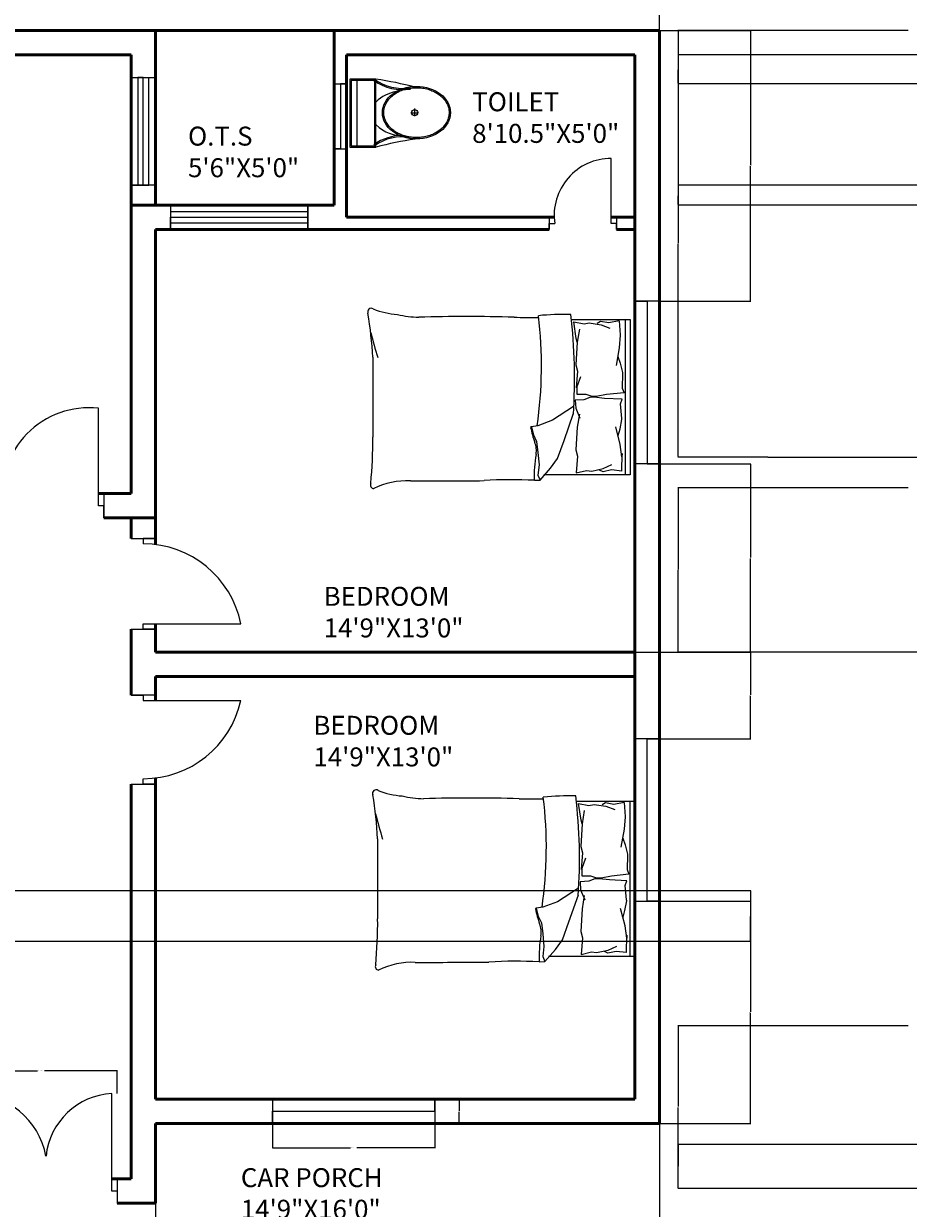
# Model space of a CAD drawing. Units: inches. Extents: x 2215 to 3724, y 1009 to 2124.
# Tile 6 of 11: x 2636 to 2963, y 1313 to 1750. Entities that reach past the tile are written whole.
import ezdxf

# ---------------------------------------------------------------- set-up
doc = ezdxf.new("R2010")
doc.units = ezdxf.units.IN
for name, color, linetype, lineweight in [('A-ANNO-DIMS', 2, 'Continuous', 18), ('A-ANNO-SYMB', 7, 'Continuous', 25), ('A-AREA-IDEN', 7, 'Continuous', 18), ('A-DOOR', 3, 'Continuous', 25), ('A-FLOR-FIXT', 9, 'Continuous', 18), ('A-FURN', 8, 'Continuous', 18), ('A-GLAZ', 4, 'Continuous', 18), ('A-WALL', 7, 'Continuous', 50)]:
    doc.layers.add(name, color=color, linetype=linetype, lineweight=lineweight)
doc.styles.get("Standard").update_dxf_attribs({"font": 'arial.ttf'})
doc.dimstyles.get("Standard").update_dxf_attribs({"dimtxt": 0.18, "dimasz": 0.18, "dimexe": 0.18, "dimexo": 0.0625, "dimgap": 0.09, "dimtad": 0, "dimtih": 1, "dimtoh": 1, "dimdec": 4, "dimzin": 0, "dimdsep": 46, "dimtxsty": 'Standard', "dimcen": 0.09, "dimadec": 0, "dimazin": 0, "dimtfac": 1, "dimtdec": 4, "dimtofl": 0, "dimtmove": 0, "dimatfit": 3, "dimfxl": 1, "dimtolj": 1, "dimtzin": 0, "dimarcsym": 0})

# ---------------------------------------------------------------- blocks, each defined once
blk = doc.blocks.new('A$C31115884')
for p, q in [((283.1, 497.7), (223.4, 497.7)), ((257.5, 466.4), (257.5, 523.2)), ((0, 200), (0, 0)), ((520, 200), (0, 200)), ((10, 190), (10, 10)), ((510, 190), (10, 190)), ((510, 10), (510, 190)), ((520, 0), (520, 200)), ((510, 54.5), (0, 54.5)), ((10, 10), (510, 10)), ((0, 0), (520, 0))]:
    blk.add_line(p, q)
blk.add_circle((255.6, 496.4), 23.6)
for centre, radius, start, end in [((2777.7, -204.6), 2807, 165.4549, 171.71327), ((-294.5, 403.3), 364.7, 324.20913, 9.34987), ((-294.5, 403.3), 374.7, 324.20913, 9.34987), ((805.8, 403.3), 364.7, 170.65013, 215.79087), ((3237, 905), 2807, 188.28673, 194.5451), ((139.5, 406.2), 293.5, 315.84364, 2.65635), ((805.8, 403.3), 374.7, 179.20365, 215.79087), ((383.6, 406.2), 293.5, 190.27735, 224.15636)]:
    blk.add_arc(centre, radius, start, end)
blk.add_ellipse((256.2, 509.9), major_axis=(0, -260.7), ratio=0.772727)
blk.add_open_spline([(256.2, 259.2), (263.1, 259.2), (270, 259.7), (287.8, 262.3), (298.7, 265.1), (319.9, 273.1), (330.2, 278.4), (350.1, 291.1), (359.7, 298.7), (377.7, 315.9), (386.2, 325.5), (401.7, 346.6), (408.8, 358.1), (421.3, 382.5), (426.8, 395.5), (435.9, 422.4), (439.5, 436.4), (444.8, 465.1), (446.5, 479.7), (447.9, 509.2), (447.6, 524), (445, 553.3), (442.7, 567.8), (436.3, 596), (432.1, 609.7), (421.9, 636), (416, 648.6), (402.5, 672.1), (395, 683), (378.6, 703), (369.8, 712.1), (351.1, 728), (341.3, 734.8), (320.9, 746.2), (310.4, 750.7), (288.9, 757.3), (278, 759.4), (256, 761), (245, 760.6), (223.1, 757.2), (212.3, 754.3), (191.1, 746.1), (180.8, 740.7), (160.9, 727.8), (151.4, 720.1), (133.5, 702.7), (125.1, 693), (109.6, 671.7), (102.6, 660.2), (90.2, 635.7), (84.9, 622.7), (76, 595.6), (72.4, 581.6), (67.2, 552.9), (65.6, 538.2), (64.4, 508.8), (64.8, 494), (67.5, 464.7), (69.9, 450.2), (76.6, 422), (80.8, 408.3), (91.1, 382.2), (97.2, 369.7), (110.8, 346.3), (118.4, 335.4), (134.8, 315.6), (143.7, 306.7), (162.4, 290.9), (172.3, 284.2), (192.8, 273), (203.3, 268.6), (224.8, 262.2), (235.8, 260.2), (249.9, 259.3), (253, 259.2), (256.2, 259.2)], degree=3, knots=[0, 0, 0, 0, 0.110105, 0.110105, 0.285049, 0.285049, 0.459994, 0.459994, 0.634938, 0.634938, 0.809882, 0.809882, 0.984827, 0.984827, 1.159771, 1.159771, 1.334715, 1.334715, 1.50966, 1.50966, 1.684604, 1.684604, 1.859549, 1.859549, 2.034493, 2.034493, 2.209437, 2.209437, 2.384382, 2.384382, 2.559326, 2.559326, 2.73427, 2.73427, 2.909215, 2.909215, 3.084159, 3.084159, 3.259103, 3.259103, 3.434048, 3.434048, 3.608992, 3.608992, 3.783936, 3.783936, 3.958881, 3.958881, 4.133825, 4.133825, 4.30877, 4.30877, 4.483714, 4.483714, 4.658658, 4.658658, 4.833603, 4.833603, 5.008547, 5.008547, 5.183491, 5.183491, 5.358436, 5.358436, 5.53338, 5.53338, 5.708324, 5.708324, 5.883269, 5.883269, 6.058213, 6.058213, 6.233158, 6.233158, 6.283185, 6.283185, 6.283185, 6.283185])
blk = doc.blocks.new('DOOR-BEDROOM-NE')
for p, q in [((0, 33.52), (0, 33.52)), ((0, 33.52), (9, 33.52)), ((9, 33.52), (4.5, 33.52)), ((4.5, 33.52), (4.5, 31.52)), ((0, 0), (9, 0)), ((4.5, 0), (4.5, 2)), ((4.5, 2), (40.5, 2)), ((9, 0), (4.5, 0))]:
    blk.add_line(p, q)
blk.add_arc((4.5, -5.19), 36.71, 11.299, 90)
blk = doc.blocks.new('DOOR-BEDROOM-SE')
for p, q in [((9, 32.82), (0, 32.82)), ((0, 32.82), (4.5, 32.82)), ((4.5, 32.82), (4.5, 30.82)), ((4.5, 30.82), (40.5, 30.82)), ((0, 0), (0, 0)), ((0, 0), (9, 0)), ((4.5, 0), (4.5, 2)), ((9, 0), (4.5, 0))]:
    blk.add_line(p, q)
blk.add_arc((4.5, 38.9), 36.9, 270, 347.3534)
blk = doc.blocks.new('DOOR-ENTRY-PAIR')
for p, q in [((2, 4.5), (2, 40.5)), ((54.26, 4.5), (54.26, 40.5)), ((0, 9), (0, 0)), ((56.26, 9), (56.26, 0)), ((0, 0), (0, 4.5)), ((0, 4.5), (2, 4.5)), ((56.26, 4.5), (54.26, 4.5))]:
    blk.add_line(p, q)
for centre, radius, start, end in [((2, 12.02), 28.48, 11.0167, 90), ((55.55, 14.8), 25.73, 92.8796, 174.0708)]:
    blk.add_arc(centre, radius, start, end)
blk = doc.blocks.new('DOOR-BATH-NE')
for p, q in [((22.84, 2.25), (22.84, 26.25)), ((0, 4.5), (0, 0)), ((24.84, 4.5), (24.84, 0)), ((0, 0), (0, 2.25)), ((0, 2.25), (2, 2.25)), ((24.84, 2.25), (22.84, 2.25)), ((24.84, 0), (24.84, 2.25))]:
    blk.add_line(p, q)
blk.add_arc((22.84, 5.2), 21.05, 90, 188.0713)
blk = doc.blocks.new('DOOR-BEDROOM-N')
for p, q in [((37.14, 4.5), (37.14, 40.5)), ((0, 9), (0, 0)), ((39.14, 9), (39.14, 0)), ((0, 0), (0, 4.5)), ((0, 4.5), (2, 4.5)), ((39.14, 4.5), (37.14, 4.5)), ((39.14, 0), (39.14, 4.5))]:
    blk.add_line(p, q)
blk.add_arc((33.66, 8.74), 31.95, 83.7441, 187.635)
blk = doc.blocks.new('WIN-60-JAMB-A')
for p, q in [((0, 9), (0, 0)), ((60, 4.5), (60, 9)), ((60, 9), (60, 0)), ((0, 0), (0, 4.5)), ((0, 4.5), (60, 4.5))]:
    blk.add_line(p, q)
blk = doc.blocks.new('WIN-OTS-E-END')
for p, q in [((0, 9), (0, 0)), ((50.62, 4.5), (50.62, 9)), ((50.62, 9), (50.62, 0)), ((50.62, 6.5), (0, 6.5)), ((0, 6.5), (0, 4.5)), ((0, 0), (0, 4.5)), ((0, 4.5), (50.62, 4.5)), ((0, 4.5), (0, 2.5)), ((50.62, 4.5), (50.62, 6.5)), ((50.62, 0), (50.62, 4.5)), ((0, 2.5), (50.62, 2.5))]:
    blk.add_line(p, q)
blk = doc.blocks.new('WIN-60-JAMB-B')
for p, q in [((9, 60), (0, 60)), ((0, 60), (4.5, 60)), ((4.5, 60), (4.5, 0)), ((4.5, 0), (0, 0)), ((0, 0), (9, 0))]:
    blk.add_line(p, q)
blk = doc.blocks.new('WIN-OTS-E-SIDE')
for p, q in [((0, 39.84), (9, 39.84)), ((3.5, 39.84), (2.5, 39.84)), ((2.5, 39.84), (2.5, 0)), ((4.5, 39.84), (3.5, 39.84)), ((4.5, 0), (4.5, 39.84)), ((6.5, 0), (6.5, 39.84)), ((9, 0), (0, 0)), ((0, 0), (4.5, 0)), ((2.5, 0), (4.5, 0)), ((4.5, 0), (6.5, 0))]:
    blk.add_line(p, q)
blk = doc.blocks.new('VENT-24-NE')
for p, q in [((0, 24), (4.5, 24)), ((4.5, 24), (2.25, 24)), ((2.25, 24), (2.25, 0)), ((2.25, 0), (0, 0)), ((0, 0), (4.5, 0))]:
    blk.add_line(p, q)
blk = doc.blocks.new('BED-DOUBLE')
for p, q in [((0, 61.46), (31.9, 61.46)), ((0, 4.17), (0, 61.46)), ((1.84, 4.17), (1.84, 61.46)), ((33.26, 63.38), (29.37, 58.94)), ((35.35, 63.48), (33.26, 63.38, 4.64)), ((34.01, 61.54), (33.26, 63.38)), ((33.63, 57.82), (34.01, 61.54)), ((3.07, 60.08), (2.95, 53.6)), ((3.07, 60.08), (6.91, 59.62)), ((9.9, 59.12), (6.69, 57.7)), ((6.91, 59.62), (10, 60.34)), ((14.18, 60.08), (9.9, 59.12)), ((10, 60.34), (11.25, 59.72)), ((16.11, 59.85), (14.18, 60.08)), ((19.87, 60.78), (16.11, 59.85)), ((19.38, 54.63), (19.87, 60.78)), ((29.37, 58.94), (26.77, 55.41)), ((34.01, 53.18), (33.63, 57.82)), ((2.95, 53.6), (3.05, 54.8)), ((3.05, 54.8), (3.68, 50.25)), ((20.05, 52.28), (19.38, 54.63)), ((26.77, 55.41), (24.36, 48.73)), ((34.56, 49.1), (34.01, 53.18)), ((3.68, 50.25), (5.3, 43.75)), ((19.54, 43.87), (20.05, 52.28)), ((24.36, 48.73), (20.84, 38.73)), ((35.68, 46.68), (34.56, 49.1)), ((3.69, 44.52), (3.04, 41.01)), ((4.4, 47), (3.69, 44.52)), ((18.74, 39.04), (19.54, 43.87)), ((36.42, 43.71), (35.68, 46.68)), ((95, 18.06), (95, 47.57)), ((3.04, 41.01), (3.07, 40.62)), ((3.07, 40.62), (3.57, 35.31)), ((20.07, 36.87), (18.53, 40.55)), ((20.84, 36.28), (28.62, 41.3)), ((28.62, 41.3), (34.01, 43.34)), ((34.01, 43.34), (36.42, 43.71)), ((3.57, 35.31), (2.99, 33.54)), ((20.25, 33.92), (20.07, 36.87)), ((2.24, 31.15), (8.66, 31.84)), ((2.94, 29.42), (2.24, 31.15)), ((2.99, 33.54), (9.43, 33.25)), ((8.66, 31.84), (12.47, 32.54)), ((9.43, 33.25), (13.28, 32.79)), ((12.47, 32.54), (14.03, 32.54)), ((13.28, 32.79), (14.84, 32.89)), ((14.03, 32.54), (16.28, 31.84)), ((14.84, 32.89), (17.04, 33.72)), ((16.28, 31.84), (19.5, 31.84)), ((17.04, 33.72), (20.25, 33.92)), ((19.5, 31.84), (19.5, 28.9)), ((2.76, 24.09), (2.94, 29.42)), ((19.5, 28.9), (18.19, 25.13)), ((19.38, 23.24), (19.87, 29.39)), ((2.76, 23.7), (2.76, 24.09)), ((3.63, 20.24), (2.76, 23.7)), ((20.05, 20.89), (19.38, 23.24)), ((4.5, 17.81), (3.63, 20.24)), ((3.98, 14.52), (5.19, 21.1)), ((19.54, 12.48), (20.05, 20.89)), ((3.63, 9.93), (3.98, 14.52)), ((3.61, 9.81), (3.63, 9.93)), ((4, 4.67), (3.61, 9.81)), ((18.74, 7.65), (19.54, 12.48)), ((19.54, 12.48), (19.92, 11.13)), ((19.92, 11.13), (20.79, 5.02)), ((3.98, 4.67), (7.79, 5.36)), ((10.74, 6.06), (7.44, 7.27)), ((7.79, 5.36), (10.91, 4.84)), ((15.07, 5.36), (10.74, 6.06)), ((10.91, 4.84), (12.12, 5.54)), ((16.98, 5.71), (15.07, 5.36)), ((20.79, 5.02), (16.98, 5.71)), ((21.71, 4.17), (0, 4.17))]:
    blk.add_line(p, q)
for centre, radius, start, end in [((82.32, 91.3), 27.65, 267.4714, 296.4681), ((94.55, 65.23), 1.32, 332.6588, 86.02), ((-7.98, 61.53), 43.38, 349.8763, 2.5657), ((43.54, 218.51), 155.25, 266.9791, 273.8365), ((81.31, -5405.34), 5469.02, 90.00217, 90.28689), ((254.49, 49.34), 159.5, 174.4998, 180.6351), ((42.04, 52.44), 7.46, 168.6608, 203.7384), ((1.78, 37.35), 35.55, 10.6617, 19.8806), ((36.49, 43.92), 0.221, 250.2464, 1.1377), ((187.4, 21.29), 154.68, 171.7845, 186.9006), ((218.25, 25.61), 197.77, 176.0865, 186.7821), ((-28.43, -20.65), 127.63, 13.3832, 17.7053), ((240.77, 25.69), 145.97, 182.9958, 189.4091), ((24.09, 102.1), 99.87, 268.7218, 275.604), ((37.37, -200.58), 203.94, 88.4762, 91.0082), ((60.68, 581.23), 578.22, 268.22771, 271.71854), ((77.34, -32.25), 35.53, 76.0648, 88.9113), ((84.25, -25.97), 28.25, 67.9751, 86.652), ((95.57, 1.3), 1.31, 236.1736, 23.4781)]:
    blk.add_arc(centre, radius, start, end)
blk = doc.blocks.new('*D31')
at = {"layer": 'A-ANNO-DIMS', "color": 0, "lineweight": -2, "transparency": 16777216}
for p, q in [((2727.98, 1343.93), (2727.98, 1334.82)), ((2787.98, 1343.93), (2787.98, 1334.82)), ((2728.16, 1335), (2756.87, 1335)), ((2787.8, 1335), (2759.1, 1335))]:
    blk.add_line(p, q, dxfattribs=at)
at = {"layer": 'A-ANNO-DIMS', "color": 0, "transparency": 16777216}
for points in [[(2728.16, 1335.03), (2728.16, 1334.97), (2727.98, 1335)], [(2787.8, 1335.03), (2787.8, 1334.97), (2787.98, 1335)]]:
    blk.add_solid(points, dxfattribs=at)
at = {"layer": 'Defpoints', "color": 0, "transparency": 16777216}
for p in [(2727.98, 1344), (2787.98, 1344), (2787.98, 1335)]:
    blk.add_point(p, dxfattribs=at)
at = {"layer": 'A-ANNO-DIMS', "color": 0, "transparency": 16777216, "insert": (2757.98, 1335), "char_height": 0.18, "attachment_point": 5}
blk.add_mtext('\\A1;WINDOW 60 TYP.', dxfattribs=at)
blk = doc.blocks.new('*D32')
at = {"layer": 'A-ANNO-DIMS', "color": 0, "lineweight": -2, "transparency": 16777216}
for p, q in [((2788.05, 1353), (2797.16, 1353)), ((2796.98, 1352.82), (2796.98, 1348.68)), ((2796.98, 1344.18), (2796.98, 1348.32)), ((2788.05, 1344), (2797.16, 1344))]:
    blk.add_line(p, q, dxfattribs=at)
at = {"layer": 'A-ANNO-DIMS', "color": 0, "transparency": 16777216}
for points in [[(2796.95, 1352.82), (2797.01, 1352.82), (2796.98, 1353)], [(2796.95, 1344.18), (2797.01, 1344.18), (2796.98, 1344)]]:
    blk.add_solid(points, dxfattribs=at)
at = {"layer": 'Defpoints', "color": 0, "transparency": 16777216}
for p in [(2787.98, 1353), (2796.98, 1353), (2787.98, 1344)]:
    blk.add_point(p, dxfattribs=at)
at = {"layer": 'A-ANNO-DIMS', "color": 0, "transparency": 16777216, "insert": (2796.98, 1348.5), "char_height": 0.18, "attachment_point": 5}
blk.add_mtext('\\A1;9 TYP.', dxfattribs=at)
blk = doc.blocks.new('*D57')
at = {"layer": 'A-ANNO-DIMS', "color": 0, "lineweight": -2, "transparency": 16777216}
for p, q in [((2614.45, 1355.05), (2614.45, 1363.61)), ((2614.63, 1363.43), (2641.27, 1363.43)), ((2670.53, 1363.43), (2643.9, 1363.43)), ((2670.71, 1355.05), (2670.71, 1363.61))]:
    blk.add_line(p, q, dxfattribs=at)
at = {"layer": 'A-ANNO-DIMS', "color": 0, "transparency": 16777216}
for points in [[(2614.63, 1363.46), (2614.63, 1363.4), (2614.45, 1363.43)], [(2670.53, 1363.46), (2670.53, 1363.4), (2670.71, 1363.43)]]:
    blk.add_solid(points, dxfattribs=at)
at = {"layer": 'Defpoints', "color": 0, "transparency": 16777216}
for p in [(2670.71, 1363.43), (2614.45, 1354.99), (2670.71, 1354.99)]:
    blk.add_point(p, dxfattribs=at)
at = {"layer": 'A-ANNO-DIMS', "color": 0, "transparency": 16777216, "insert": (2642.58, 1363.43), "char_height": 0.18, "attachment_point": 5}
blk.add_mtext('\\A1;ENTRY PAIR 56 TYP.', dxfattribs=at)
blk = doc.blocks.new('*D87')
at = {"layer": 'A-ANNO-DIMS', "color": 0, "lineweight": -2, "transparency": 16777216}
for p, q in [((2312.84, 1747.56), (2312.84, 1781.28)), ((2313.02, 1781.1), (2591.55, 1781.1)), ((2870.66, 1781.1), (2592.13, 1781.1)), ((2870.84, 1747.56), (2870.84, 1781.28))]:
    blk.add_line(p, q, dxfattribs=at)
at = {"layer": 'A-ANNO-DIMS', "color": 0, "transparency": 16777216}
for points in [[(2313.02, 1781.13), (2313.02, 1781.07), (2312.84, 1781.1)], [(2870.66, 1781.13), (2870.66, 1781.07), (2870.84, 1781.1)]]:
    blk.add_solid(points, dxfattribs=at)
at = {"layer": 'Defpoints', "color": 0, "transparency": 16777216}
for p in [(2870.84, 1781.1), (2312.84, 1747.5), (2870.84, 1747.5)]:
    blk.add_point(p, dxfattribs=at)
at = {"layer": 'A-ANNO-DIMS', "color": 0, "transparency": 16777216, "insert": (2591.84, 1781.1), "char_height": 0.18, "attachment_point": 5}
blk.add_mtext('\\A1;558', dxfattribs=at)
blk = doc.blocks.new('*D90')
at = {"layer": 'A-ANNO-DIMS', "color": 0, "lineweight": -2, "transparency": 16777216}
for p, q in [((2962.68, 1380.03), (2877.61, 1380.03)), ((2877.79, 1379.85), (2877.79, 1350.2)), ((2877.79, 1320.18), (2877.79, 1349.83)), ((2971.68, 1320), (2877.61, 1320))]:
    blk.add_line(p, q, dxfattribs=at)
at = {"layer": 'A-ANNO-DIMS', "color": 0, "transparency": 16777216}
for points in [[(2877.76, 1379.85), (2877.82, 1379.85), (2877.79, 1380.03)], [(2877.76, 1320.18), (2877.82, 1320.18), (2877.79, 1320)]]:
    blk.add_solid(points, dxfattribs=at)
at = {"layer": 'Defpoints', "color": 0, "transparency": 16777216}
for p in [(2877.79, 1380.03), (2962.74, 1380.03), (2971.74, 1320)]:
    blk.add_point(p, dxfattribs=at)
at = {"layer": 'A-ANNO-DIMS', "color": 0, "transparency": 16777216, "insert": (2877.79, 1350.01), "char_height": 0.18, "attachment_point": 5}
blk.add_mtext('\\A1;60.03', dxfattribs=at)
blk = doc.blocks.new('*D91')
at = {"layer": 'A-ANNO-DIMS', "color": 0, "lineweight": -2, "transparency": 16777216}
for p, q in [((2962.68, 1578.61), (2877.61, 1578.61)), ((2877.79, 1578.43), (2877.79, 1548.49)), ((2877.79, 1518.18), (2877.79, 1548.12)), ((2971.68, 1518), (2877.61, 1518))]:
    blk.add_line(p, q, dxfattribs=at)
at = {"layer": 'A-ANNO-DIMS', "color": 0, "transparency": 16777216}
for points in [[(2877.76, 1578.43), (2877.82, 1578.43), (2877.79, 1578.61)], [(2877.76, 1518.18), (2877.82, 1518.18), (2877.79, 1518)]]:
    blk.add_solid(points, dxfattribs=at)
at = {"layer": 'Defpoints', "color": 0, "transparency": 16777216}
for p in [(2877.79, 1578.61), (2962.74, 1578.61), (2971.74, 1518)]:
    blk.add_point(p, dxfattribs=at)
at = {"layer": 'A-ANNO-DIMS', "color": 0, "transparency": 16777216, "insert": (2877.79, 1548.3), "char_height": 0.18, "attachment_point": 5}
blk.add_mtext('\\A1;60.61', dxfattribs=at)
blk = doc.blocks.new('*D92')
at = {"layer": 'A-ANNO-DIMS', "color": 0, "lineweight": -2, "transparency": 16777216}
for p, q in [((2870.9, 1747.5), (2904.62, 1747.5)), ((2904.44, 1747.32), (2904.44, 1697.7)), ((2904.44, 1647.72), (2904.44, 1697.34)), ((2870.9, 1647.54), (2904.62, 1647.54))]:
    blk.add_line(p, q, dxfattribs=at)
at = {"layer": 'A-ANNO-DIMS', "color": 0, "transparency": 16777216}
for points in [[(2904.41, 1747.32), (2904.47, 1747.32), (2904.44, 1747.5)], [(2904.41, 1647.72), (2904.47, 1647.72), (2904.44, 1647.54)]]:
    blk.add_solid(points, dxfattribs=at)
at = {"layer": 'Defpoints', "color": 0, "transparency": 16777216}
for p in [(2870.84, 1747.5), (2904.44, 1747.5), (2870.84, 1647.54)]:
    blk.add_point(p, dxfattribs=at)
at = {"layer": 'A-ANNO-DIMS', "color": 0, "transparency": 16777216, "insert": (2904.44, 1697.52), "char_height": 0.18, "attachment_point": 5}
blk.add_mtext('\\A1;99.96', dxfattribs=at)
blk = doc.blocks.new('*D93')
at = {"layer": 'A-ANNO-DIMS', "color": 0, "lineweight": -2, "transparency": 16777216}
for p, q in [((2870.9, 1425.98), (2904.62, 1425.98)), ((2904.44, 1425.8), (2904.44, 1385.17)), ((2904.44, 1344.18), (2904.44, 1384.8)), ((2870.9, 1344), (2904.62, 1344))]:
    blk.add_line(p, q, dxfattribs=at)
at = {"layer": 'A-ANNO-DIMS', "color": 0, "transparency": 16777216}
for points in [[(2904.41, 1425.8), (2904.47, 1425.8), (2904.44, 1425.98)], [(2904.41, 1344.18), (2904.47, 1344.18), (2904.44, 1344)]]:
    blk.add_solid(points, dxfattribs=at)
at = {"layer": 'Defpoints', "color": 0, "transparency": 16777216}
for p in [(2870.84, 1425.98), (2904.44, 1425.98), (2870.84, 1344)]:
    blk.add_point(p, dxfattribs=at)
at = {"layer": 'A-ANNO-DIMS', "color": 0, "transparency": 16777216, "insert": (2904.44, 1384.99), "char_height": 0.18, "attachment_point": 5}
blk.add_mtext('\\A1;81.98', dxfattribs=at)
blk = doc.blocks.new('*D94')
at = {"layer": 'A-ANNO-DIMS', "color": 0, "lineweight": -2, "transparency": 16777216}
for p, q in [((2861.9, 1518), (2904.62, 1518)), ((2904.44, 1517.82), (2904.44, 1502.17)), ((2904.44, 1486.16), (2904.44, 1501.8)), ((2870.9, 1485.98), (2904.62, 1485.98))]:
    blk.add_line(p, q, dxfattribs=at)
at = {"layer": 'A-ANNO-DIMS', "color": 0, "transparency": 16777216}
for points in [[(2904.41, 1517.82), (2904.47, 1517.82), (2904.44, 1518)], [(2904.41, 1486.16), (2904.47, 1486.16), (2904.44, 1485.98)]]:
    blk.add_solid(points, dxfattribs=at)
at = {"layer": 'Defpoints', "color": 0, "transparency": 16777216}
for p in [(2861.84, 1518), (2904.44, 1518), (2870.84, 1485.98)]:
    blk.add_point(p, dxfattribs=at)
at = {"layer": 'A-ANNO-DIMS', "color": 0, "transparency": 16777216, "insert": (2904.44, 1501.99), "char_height": 0.18, "attachment_point": 5}
blk.add_mtext('\\A1;32.02', dxfattribs=at)
blk = doc.blocks.new('*D95')
at = {"layer": 'A-ANNO-DIMS', "color": 0, "lineweight": -2, "transparency": 16777216}
for p, q in [((2870.9, 1587.54), (2904.62, 1587.54)), ((2904.44, 1587.36), (2904.44, 1552.95)), ((2904.44, 1518.18), (2904.44, 1552.59)), ((2861.9, 1518), (2904.62, 1518))]:
    blk.add_line(p, q, dxfattribs=at)
at = {"layer": 'A-ANNO-DIMS', "color": 0, "transparency": 16777216}
for points in [[(2904.41, 1587.36), (2904.47, 1587.36), (2904.44, 1587.54)], [(2904.41, 1518.18), (2904.47, 1518.18), (2904.44, 1518)]]:
    blk.add_solid(points, dxfattribs=at)
at = {"layer": 'Defpoints', "color": 0, "transparency": 16777216}
for p in [(2870.84, 1587.54), (2904.44, 1587.54), (2861.84, 1518)]:
    blk.add_point(p, dxfattribs=at)
at = {"layer": 'A-ANNO-DIMS', "color": 0, "transparency": 16777216, "insert": (2904.44, 1552.77), "char_height": 0.18, "attachment_point": 5}
blk.add_mtext('\\A1;69.54', dxfattribs=at)
blk = doc.blocks.new('*D96')
at = {"layer": 'A-ANNO-DIMS', "color": 0, "lineweight": -2, "transparency": 16777216}
for p, q in [((3520.74, 1343.93), (3520.74, 1118.67)), ((2962.74, 1151.93), (2962.74, 1118.67)), ((2962.92, 1118.85), (3241.45, 1118.85)), ((3520.56, 1118.85), (3242.03, 1118.85))]:
    blk.add_line(p, q, dxfattribs=at)
at = {"layer": 'A-ANNO-DIMS', "color": 0, "transparency": 16777216}
for points in [[(2962.92, 1118.88), (2962.92, 1118.82), (2962.74, 1118.85)], [(3520.56, 1118.88), (3520.56, 1118.82), (3520.74, 1118.85)]]:
    blk.add_solid(points, dxfattribs=at)
at = {"layer": 'Defpoints', "color": 0, "transparency": 16777216}
for p in [(3520.74, 1344), (2962.74, 1152), (3520.74, 1118.85)]:
    blk.add_point(p, dxfattribs=at)
at = {"layer": 'A-ANNO-DIMS', "color": 0, "transparency": 16777216, "insert": (3241.74, 1118.85), "char_height": 0.18, "attachment_point": 5}
blk.add_mtext('\\A1;558', dxfattribs=at)
blk = doc.blocks.new('*D99')
at = {"layer": 'A-ANNO-DIMS', "color": 0, "lineweight": -2, "transparency": 16777216}
for p, q in [((2684.84, 1343.93), (2684.84, 1118.22)), ((2609.84, 1151.93), (2609.84, 1118.22)), ((2610.02, 1118.4), (2647.12, 1118.4)), ((2684.66, 1118.4), (2647.56, 1118.4))]:
    blk.add_line(p, q, dxfattribs=at)
at = {"layer": 'A-ANNO-DIMS', "color": 0, "transparency": 16777216}
for points in [[(2610.02, 1118.43), (2610.02, 1118.37), (2609.84, 1118.4)], [(2684.66, 1118.43), (2684.66, 1118.37), (2684.84, 1118.4)]]:
    blk.add_solid(points, dxfattribs=at)
at = {"layer": 'Defpoints', "color": 0, "transparency": 16777216}
for p in [(2684.84, 1344), (2609.84, 1152), (2684.84, 1118.4)]:
    blk.add_point(p, dxfattribs=at)
at = {"layer": 'A-ANNO-DIMS', "color": 0, "transparency": 16777216, "insert": (2647.34, 1118.4), "char_height": 0.18, "attachment_point": 5}
blk.add_mtext('\\A1;75', dxfattribs=at)
blk = doc.blocks.new('*D100')
at = {"layer": 'A-ANNO-DIMS', "color": 0, "lineweight": -2, "transparency": 16777216}
for p, q in [((2684.84, 1343.93), (2684.84, 1118.22)), ((2870.84, 1343.93), (2870.84, 1118.22)), ((2685.02, 1118.4), (2777.56, 1118.4)), ((2870.66, 1118.4), (2778.12, 1118.4))]:
    blk.add_line(p, q, dxfattribs=at)
at = {"layer": 'A-ANNO-DIMS', "color": 0, "transparency": 16777216}
for points in [[(2685.02, 1118.43), (2685.02, 1118.37), (2684.84, 1118.4)], [(2870.66, 1118.43), (2870.66, 1118.37), (2870.84, 1118.4)]]:
    blk.add_solid(points, dxfattribs=at)
at = {"layer": 'Defpoints', "color": 0, "transparency": 16777216}
for p in [(2684.84, 1344), (2870.84, 1344), (2870.84, 1118.4)]:
    blk.add_point(p, dxfattribs=at)
at = {"layer": 'A-ANNO-DIMS', "color": 0, "transparency": 16777216, "insert": (2777.84, 1118.4), "char_height": 0.18, "attachment_point": 5}
blk.add_mtext('\\A1;186', dxfattribs=at)
blk = doc.blocks.new('*D101')
at = {"layer": 'A-ANNO-DIMS', "color": 0, "lineweight": -2, "transparency": 16777216}
for p, q in [((2962.68, 1747.5), (2877.61, 1747.5)), ((2877.79, 1747.32), (2877.79, 1668.93)), ((2877.79, 1590.18), (2877.79, 1668.57)), ((2910.88, 1590), (2877.61, 1590))]:
    blk.add_line(p, q, dxfattribs=at)
at = {"layer": 'A-ANNO-DIMS', "color": 0, "transparency": 16777216}
for points in [[(2877.76, 1747.32), (2877.82, 1747.32), (2877.79, 1747.5)], [(2877.76, 1590.18), (2877.82, 1590.18), (2877.79, 1590)]]:
    blk.add_solid(points, dxfattribs=at)
at = {"layer": 'Defpoints', "color": 0, "transparency": 16777216}
for p in [(2877.79, 1747.5), (2962.74, 1747.5), (2910.94, 1590)]:
    blk.add_point(p, dxfattribs=at)
at = {"layer": 'A-ANNO-DIMS', "color": 0, "transparency": 16777216, "insert": (2877.79, 1668.75), "char_height": 0.18, "attachment_point": 5}
blk.add_mtext('\\A1;157.5', dxfattribs=at)
blk = doc.blocks.new('*D105')
at = {"layer": 'A-ANNO-DIMS', "color": 0, "lineweight": -2, "transparency": 16777216}
for p, q in [((2591.12, 1430.02), (2904.62, 1430.02)), ((2904.44, 1429.84), (2904.44, 1420.79)), ((2904.44, 1411.39), (2904.44, 1420.43)), ((2591.12, 1411.21), (2904.62, 1411.21))]:
    blk.add_line(p, q, dxfattribs=at)
at = {"layer": 'A-ANNO-DIMS', "color": 0, "transparency": 16777216}
for points in [[(2904.41, 1429.84), (2904.47, 1429.84), (2904.44, 1430.02)], [(2904.41, 1411.39), (2904.47, 1411.39), (2904.44, 1411.21)]]:
    blk.add_solid(points, dxfattribs=at)
at = {"layer": 'Defpoints', "color": 0, "transparency": 16777216}
for p in [(2591.06, 1430.02), (2904.44, 1430.02), (2591.06, 1411.21)]:
    blk.add_point(p, dxfattribs=at)
at = {"layer": 'A-ANNO-DIMS', "color": 0, "transparency": 16777216, "insert": (2904.44, 1420.61), "char_height": 0.18, "attachment_point": 5}
blk.add_mtext('\\A1;18.81', dxfattribs=at)
blk = doc.blocks.new('*D124')
at = {"layer": 'A-ANNO-DIMS', "color": 0, "lineweight": -2, "transparency": 16777216}
for p, q in [((3334.68, 1690.31), (2877.61, 1690.31)), ((2877.79, 1690.13), (2877.79, 1686.83)), ((2877.79, 1683.18), (2877.79, 1686.47)), ((3334.68, 1683), (2877.61, 1683))]:
    blk.add_line(p, q, dxfattribs=at)
at = {"layer": 'A-ANNO-DIMS', "color": 0, "transparency": 16777216}
for points in [[(2877.76, 1690.13), (2877.82, 1690.13), (2877.79, 1690.31)], [(2877.76, 1683.18), (2877.82, 1683.18), (2877.79, 1683)]]:
    blk.add_solid(points, dxfattribs=at)
at = {"layer": 'Defpoints', "color": 0, "transparency": 16777216}
for p in [(2877.79, 1690.31), (3334.74, 1690.31), (3334.74, 1683)]:
    blk.add_point(p, dxfattribs=at)
at = {"layer": 'A-ANNO-DIMS', "color": 0, "transparency": 16777216, "insert": (2877.79, 1686.65), "char_height": 0.18, "attachment_point": 5}
blk.add_mtext('\\A1;7.31', dxfattribs=at)
blk = doc.blocks.new('*D125')
at = {"layer": 'A-ANNO-DIMS', "color": 0, "lineweight": -2, "transparency": 16777216}
for p, q in [((3405.18, 1738.5), (2877.61, 1738.5)), ((2877.79, 1738.32), (2877.79, 1733.33)), ((2877.79, 1727.97), (2877.79, 1732.96)), ((3405.18, 1727.79), (2877.61, 1727.79))]:
    blk.add_line(p, q, dxfattribs=at)
at = {"layer": 'A-ANNO-DIMS', "color": 0, "transparency": 16777216}
for points in [[(2877.76, 1738.32), (2877.82, 1738.32), (2877.79, 1738.5)], [(2877.76, 1727.97), (2877.82, 1727.97), (2877.79, 1727.79)]]:
    blk.add_solid(points, dxfattribs=at)
at = {"layer": 'Defpoints', "color": 0, "transparency": 16777216}
for p in [(2877.79, 1738.5), (3405.24, 1738.5), (3405.24, 1727.79)]:
    blk.add_point(p, dxfattribs=at)
at = {"layer": 'A-ANNO-DIMS', "color": 0, "transparency": 16777216, "insert": (2877.79, 1733.14), "char_height": 0.18, "attachment_point": 5}
blk.add_mtext('\\A1;10.706', dxfattribs=at)
blk = doc.blocks.new('*D126')
at = {"layer": 'A-ANNO-DIMS', "color": 0, "lineweight": -2, "transparency": 16777216}
for p, q in [((2990.35, 1336.24), (2877.61, 1336.24)), ((2877.79, 1336.06), (2877.79, 1328.3)), ((2877.79, 1320.18), (2877.79, 1327.94)), ((2971.68, 1320), (2877.61, 1320))]:
    blk.add_line(p, q, dxfattribs=at)
at = {"layer": 'A-ANNO-DIMS', "color": 0, "transparency": 16777216}
for points in [[(2877.76, 1336.06), (2877.82, 1336.06), (2877.79, 1336.24)], [(2877.76, 1320.18), (2877.82, 1320.18), (2877.79, 1320)]]:
    blk.add_solid(points, dxfattribs=at)
at = {"layer": 'Defpoints', "color": 0, "transparency": 16777216}
for p in [(2877.79, 1336.24), (2990.42, 1336.24), (2971.74, 1320)]:
    blk.add_point(p, dxfattribs=at)
at = {"layer": 'A-ANNO-DIMS', "color": 0, "transparency": 16777216, "insert": (2877.79, 1328.12), "char_height": 0.18, "attachment_point": 5}
blk.add_mtext('\\A1;16.24', dxfattribs=at)

msp = doc.modelspace()

# ---------------------------------------------------------------- linework, layer by layer
at = {"layer": 'A-ANNO-SYMB'}
msp.add_line((2910.9414, 1589.9969), (3556.9429, 1589.9969), dxfattribs=at)
at = {"layer": 'A-WALL'}
for p, q in [((2312.841, 1747.4969), (2870.841, 1747.4969)), ((2684.841, 1747.4969), (2684.841, 1682.9969)), ((2750.841, 1747.4969), (2750.841, 1682.9969)), ((2870.841, 1747.4969), (2870.841, 1343.9969)), ((2507.841, 1738.4969), (2675.841, 1738.4969)), ((2675.841, 1738.4969), (2675.841, 1576.4969)), ((2755.341, 1738.4969), (2755.341, 1678.4969)), ((2755.341, 1738.4969), (2861.841, 1738.4969)), ((2861.841, 1738.4969), (2861.841, 1352.9969)), ((2684.841, 1682.9969), (2675.841, 1682.9969)), ((2750.841, 1682.9969), (2684.841, 1682.9969)), ((2755.341, 1678.4969), (2832.0184, 1678.4969)), ((2853.0518, 1678.4969), (2861.841, 1678.4969)), ((2684.841, 1673.9969), (2830.2151, 1673.9969)), ((2684.841, 1673.9969), (2684.841, 1567.4969)), ((2855.0518, 1673.9969), (2861.841, 1673.9969)), ((2663.739, 1576.4969), (2675.841, 1576.4969)), ((2663.739, 1576.4969), (2675.841, 1576.4969)), ((2663.739, 1576.4969), (2675.841, 1576.4969)), ((2665.739, 1567.4969), (2684.841, 1567.4969)), ((2675.841, 1567.4969), (2675.841, 1559.9139)), ((2684.841, 1567.4969), (2684.841, 1557.637)), ((2675.841, 1526.3952), (2675.841, 1502.0746)), ((2684.841, 1528.3952), (2684.841, 1517.9969)), ((2684.841, 1517.9969), (2861.841, 1517.9969)), ((2861.841, 1508.9969), (2684.841, 1508.9969)), ((2684.841, 1508.9969), (2684.841, 1500.0746)), ((2684.841, 1471.5327), (2684.841, 1352.9969)), ((2675.841, 1469.2572), (2675.841, 1343.9969)), ((2861.841, 1352.9969), (2684.841, 1352.9969)), ((2675.841, 1343.9969), (2675.841, 1323.4864)), ((2870.841, 1343.9969), (2684.841, 1343.9969)), ((2684.841, 1318.9864), (2684.841, 1343.9969)), ((2668.7119, 1323.4864), (2675.841, 1323.4864)), ((2684.841, 1314.4864), (2684.841, 1318.9864)), ((2670.7119, 1314.4864), (2684.841, 1314.4864))]:
    msp.add_line(p, q, dxfattribs=at)

# ---------------------------------------------------------------- block references
at = {"layer": 'A-DOOR'}
for name, p in [('DOOR-BATH-NE', (2830.215, 1673.997)), ('DOOR-BEDROOM-N', (2626.595, 1567.497)), ('DOOR-BEDROOM-NE', (2675.841, 1526.395)), ('DOOR-BEDROOM-SE', (2675.841, 1469.257)), ('DOOR-ENTRY-PAIR', (2614.453, 1314.486))]:
    msp.add_blockref(name, p, dxfattribs=at)
at = {"layer": 'A-FLOR-FIXT', "xscale": 0.048164045903398, "yscale": 0.048164045903398, "zscale": 0.048164045903398, "rotation": 270}
msp.add_blockref('A$C31115884', (2756.5987, 1729.4707), dxfattribs=at)
at = {"layer": 'A-FURN', "rotation": 180}
for p in [(2860.0389, 1644.8859), (2861.8405, 1467.1232)]:
    msp.add_blockref('BED-DOUBLE', p, dxfattribs=at)
at = {"layer": 'A-GLAZ'}
for name, p in [('WIN-OTS-E-SIDE', (2675.841, 1690.308)), ('VENT-24-NE', (2750.841, 1703.791)), ('WIN-OTS-E-END', (2690.399, 1673.997)), ('WIN-60-JAMB-A', (2727.9845, 1343.997))]:
    msp.add_blockref(name, p, dxfattribs=at)
for name, p, rotation in [('WIN-60-JAMB-A', (2861.8411, 1647.5401), 270.0000000000003), ('WIN-60-JAMB-B', (2870.841, 1485.9762), 180)]:
    msp.add_blockref(name, p, dxfattribs=dict(at, rotation=rotation))

# ---------------------------------------------------------------- texts
at = {"layer": 'A-AREA-IDEN', "char_height": 7, "attachment_point": 1}
for s, width, insert in [('TOILET\\P8\'10.5"X5\'0"', 103.316377, (2801.7496, 1724.645)), ('O.T.S\\P5\'6"X5\'0"', 96.561707, (2696.8371, 1711.9653)), ('BEDROOM\\P14\'9"X13\'0"', 149.078038, (2746.9117, 1542.0721)), ('BEDROOM\\P14\'9"X13\'0"', 137.949197, (2743.1303, 1494.4582)), ('CAR PORCH\\P14\'9"X16\'0"', 75.160792, (2716.3442, 1327.4605))]:
    msp.add_mtext_dynamic_manual_height_columns(s, width=width, gutter_width=12.5, heights=[0], dxfattribs=dict(at, insert=insert))

# ---------------------------------------------------------------- dimensions: what is measured, and where the dimension line sits
at = {"layer": 'A-ANNO-DIMS'}
for base, p1, p2, picture, middle in [((2870.841, 1781.0969), (2312.841, 1747.4969), (2870.841, 1747.4969), '*D87', (2591.841, 1781.0969)), ((2684.841, 1118.3969), (2609.841, 1151.9969), (2684.841, 1343.9969), '*D99', (2647.341, 1118.3969)), ((2870.841, 1118.3969), (2684.841, 1343.9969), (2870.841, 1343.9969), '*D100', (2777.841, 1118.3969)), ((3520.7432, 1118.8469), (2962.7432, 1151.9969), (3520.7432, 1343.9969), '*D96', (3241.7432, 1118.8469))]:
    dim = msp.add_linear_dim(base=base, p1=p1, p2=p2, dimstyle='Standard', override={"dimdec": 0, "dimlfac": 1, "dimrnd": 0, "dimzin": 0, "dimdsep": 46, "dimlunit": 2}, dxfattribs=at)
    dim.commit()
    dim.dimension.update_dxf_attribs({"geometry": picture, "text_midpoint": middle})
for base, p1, p2, override, picture, middle in [((2904.441, 1747.4969), (2870.841, 1647.5399), (2870.841, 1747.4969), {"dimdec": 2, "dimlfac": 1, "dimrnd": 0, "dimzin": 0, "dimdsep": 46, "dimlunit": 2}, '*D92', (2904.441, 1697.5184)), ((2877.7914, 1747.4969), (2910.9414, 1589.9969), (2962.7432, 1747.4969), {"dimdec": 1, "dimlfac": 1, "dimrnd": 0, "dimzin": 0, "dimdsep": 46, "dimlunit": 2}, '*D101', (2877.7914, 1668.7469)), ((2877.7914, 1738.4969), (3405.2432, 1727.7909), (3405.2432, 1738.4969), {"dimdec": 3, "dimlfac": 1, "dimrnd": 0, "dimzin": 0, "dimdsep": 46, "dimlunit": 2}, '*D125', (2877.7914, 1733.1439)), ((2877.7914, 1690.3077), (3334.7432, 1682.9969), (3334.7432, 1690.3077), {"dimdec": 2, "dimlfac": 1, "dimrnd": 0, "dimzin": 0, "dimdsep": 46, "dimlunit": 2}, '*D124', (2877.7914, 1686.6523)), ((2904.441, 1587.5399), (2861.841, 1517.9969), (2870.841, 1587.5399), {"dimdec": 2, "dimlfac": 1, "dimrnd": 0, "dimzin": 0, "dimdsep": 46, "dimlunit": 2}, '*D95', (2904.441, 1552.7684)), ((2877.7914, 1578.6109), (2971.7432, 1517.9969), (2962.7432, 1578.6109), {"dimdec": 2, "dimlfac": 1, "dimrnd": 0, "dimzin": 0, "dimdsep": 46, "dimlunit": 2}, '*D91', (2877.7914, 1548.3039)), ((2904.441, 1517.9969), (2870.841, 1485.9758), (2861.841, 1517.9969), {"dimdec": 2, "dimlfac": 1, "dimrnd": 0, "dimzin": 0, "dimdsep": 46, "dimlunit": 2}, '*D94', (2904.441, 1501.9864)), ((2904.441, 1430.018), (2591.0617, 1411.2079), (2591.0617, 1430.018), {"dimdec": 2, "dimlfac": 1, "dimrnd": 0, "dimzin": 0, "dimdsep": 46, "dimlunit": 2}, '*D105', (2904.441, 1420.6129)), ((2904.441, 1425.9758), (2870.841, 1343.9969), (2870.841, 1425.9758), {"dimdec": 2, "dimlfac": 1, "dimrnd": 0, "dimzin": 0, "dimdsep": 46, "dimlunit": 2}, '*D93', (2904.441, 1384.9864)), ((2877.7914, 1380.0306), (2971.7432, 1319.9969), (2962.7432, 1380.0306), {"dimdec": 2, "dimlfac": 1, "dimrnd": 0, "dimzin": 0, "dimdsep": 46, "dimlunit": 2}, '*D90', (2877.7914, 1350.0138)), ((2877.7914, 1336.2381), (2971.7432, 1319.9969), (2990.4162, 1336.2381), {"dimdec": 2, "dimlfac": 1, "dimrnd": 0, "dimzin": 0, "dimdsep": 46, "dimlunit": 2}, '*D126', (2877.7914, 1328.1175))]:
    dim = msp.add_linear_dim(base=base, p1=p1, p2=p2, angle=90, dimstyle='Standard', override=override, dxfattribs=at)
    dim.commit()
    dim.dimension.update_dxf_attribs({"geometry": picture, "text_midpoint": middle})
for base, p1, p2, text, picture, middle in [((2670.7119, 1363.4253), (2614.4526, 1354.9864), (2670.7119, 1354.9864), 'ENTRY PAIR <> TYP.', '*D57', (2642.5822, 1363.4253)), ((2787.9846, 1334.9969), (2727.9846, 1343.9969), (2787.9846, 1343.9969), 'WINDOW <> TYP.', '*D31', (2757.9846, 1334.9969))]:
    dim = msp.add_linear_dim(base=base, p1=p1, p2=p2, text=text, dimstyle='Standard', override={"dimdec": 0, "dimlfac": 1, "dimrnd": 0, "dimzin": 0, "dimdsep": 46, "dimlunit": 2}, dxfattribs=at)
    dim.commit()
    dim.dimension.update_dxf_attribs({"geometry": picture, "text_midpoint": middle})
dim = msp.add_linear_dim(base=(2796.9846, 1352.9969), p1=(2787.9846, 1343.9969), p2=(2787.9846, 1352.9969), angle=90, text='<> TYP.', dimstyle='Standard', override={"dimdec": 0, "dimlfac": 1, "dimrnd": 0, "dimzin": 0, "dimdsep": 46, "dimlunit": 2}, dxfattribs=at)
dim.commit()
dim.dimension.update_dxf_attribs({"geometry": '*D32', "text_midpoint": (2796.9846, 1348.4969)})

doc.saveas('drawing.dxf')
